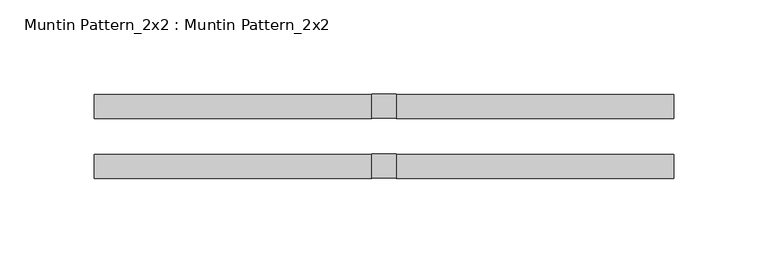
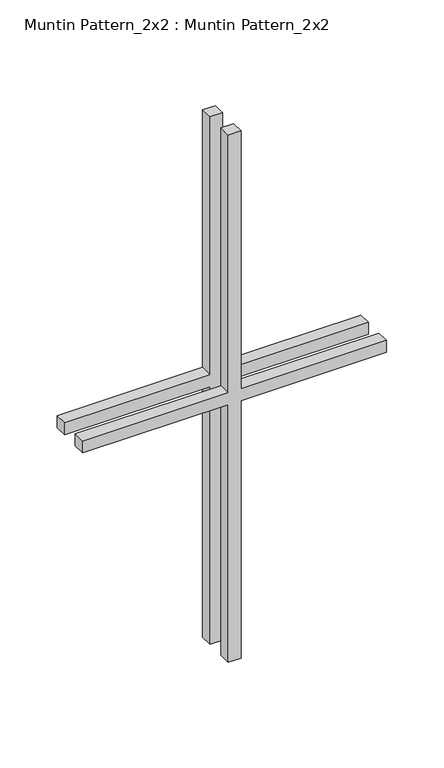
"""IFC4 building model written with IfcOpenShell, lengths in millimetres: proxy geometry, Muntin Pattern_2x2 : Muntin Pattern_2x2."""

from ifc_helpers import new_model, si_unit, frame, origin, place, context, project, spatial, polyline, outline, extrude, source, transform, mapped, element, save


def muntin_pattern_2x2_muntin_pattern_2x2_cd1db81d(model_context):
    return source(origin(), model_context, "Body", "SweptSolid", [
        extrude(outline(polyline([(287.3375, -6.35), (287.3375, -153.19375), (274.6375, -153.19375), (274.6375, -6.35), (0.0, -6.35), (0.0, 6.35), (274.6375, 6.35), (274.6375, 153.19375), (287.3375, 153.19375), (287.3375, 6.35), (561.975, 6.35), (561.975, -6.35), (287.3375, -6.35)])), frame((0.0, 9.525, 0.0), z_axis=(0.0, 1.0, 0.0), x_axis=(0.0, 0.0, 1.0)), (0.0, 0.0, 1.0), 12.7),
        extrude(outline(polyline([(287.3375, -6.35), (287.3375, -153.19375), (274.6375, -153.19375), (274.6375, -6.35), (0.0, -6.35), (0.0, 6.35), (274.6375, 6.35), (274.6375, 153.19375), (287.3375, 153.19375), (287.3375, 6.35), (561.975, 6.35), (561.975, -6.35), (287.3375, -6.35)])), frame((0.0, -22.225, 0.0), z_axis=(0.0, 1.0, 0.0), x_axis=(0.0, 0.0, 1.0)), (0.0, 0.0, 1.0), 12.7),
    ])


if __name__ == "__main__":
    model = new_model("IFC4")
    model_context = context("Model", 3, world=origin())
    ifc_project = project(units=[si_unit("LENGTHUNIT", "METRE", prefix="MILLI")], contexts=[model_context])
    site = spatial("IfcSite", under=ifc_project)
    building = spatial("IfcBuilding", under=site)
    placement = place(None, origin())
    muntin_pattern_2x2_muntin_pattern_2x2_shape = muntin_pattern_2x2_muntin_pattern_2x2_cd1db81d(model_context)
    element("IfcBuildingElementProxy", 1, Name="Muntin Pattern_2x2 : Muntin Pattern_2x2", ObjectType="Muntin Pattern_2x2 : Muntin Pattern_2x2", at=placement, inside=building, context=model_context, shape_type="MappedRepresentation", body=[
        mapped(muntin_pattern_2x2_muntin_pattern_2x2_shape, transform((0.0, 0.0, 0.0), x_axis=(1.0, 0.0, 0.0), y_axis=(0.0, 1.0, 0.0), z_axis=(0.0, 0.0, 1.0))),
    ])
    save(model, "model.ifc")

# Revit data of these elements
# Type "Muntin Pattern_2x2 : Muntin Pattern_2x2"
#   Width [instance default] = 4' - 0"
#   Thickness = 0' - 0 1/2"
#   Height [instance default] = 4' - 0"
#   Distance = 0' - 0 3/4"
#   Interior Material [instance default] = none
#   Exterior Material [instance default] = none
#   Default Elevation = 0
# Element 1 (IfcBuildingElementProxy, "Muntin Pattern_2x2 : Muntin Pattern_2x2")
#   Width = 1' - 0 1/16"
#   Height = 1' - 10 1/8"
#   Interior Material = Wood - Stained
#   Exterior Material = Clad - White
#   Materials on its faces: "Clad - White", "Wood - Stained"
# Materials
#   "Clad - White": class "Wood", colour RGB 242 242 238, transparency 0, Cost = 0
#   "Wood - Stained": class "Wood", colour RGB 224 178 126, transparency 0, Cost = 0
